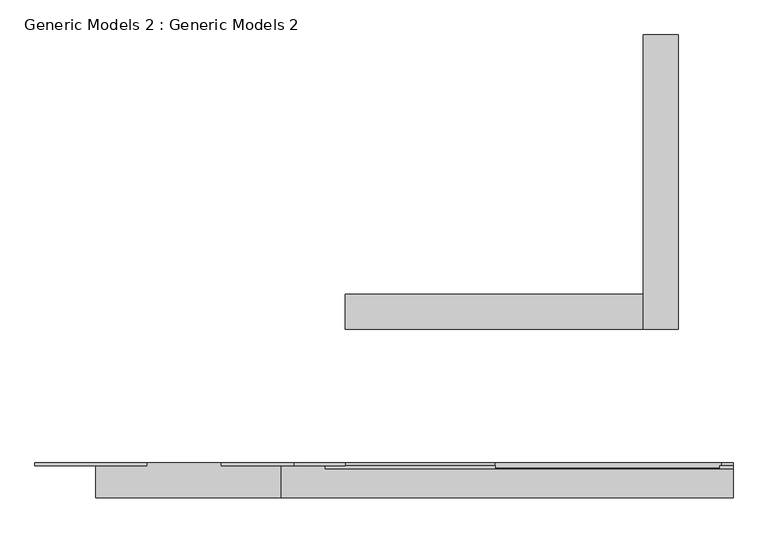
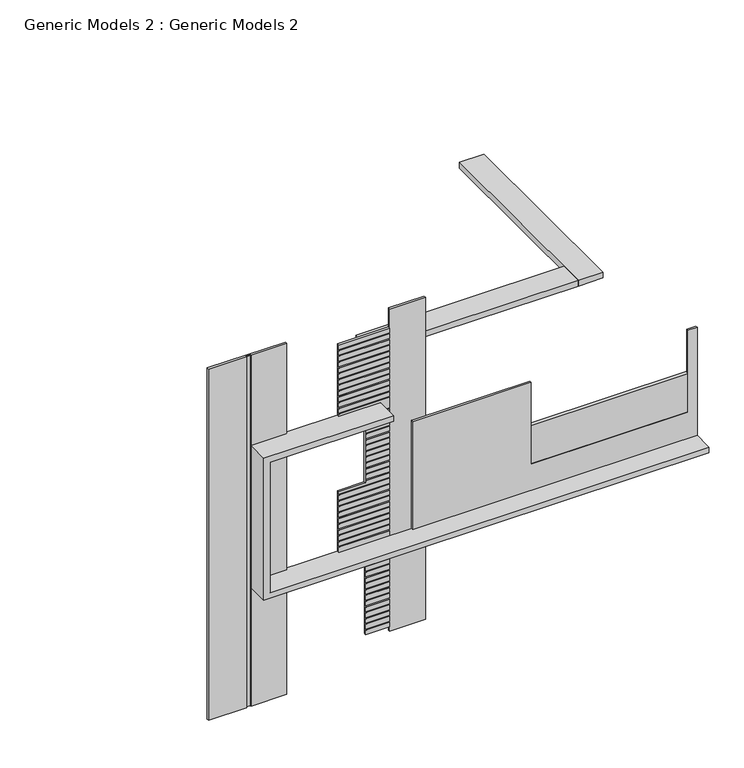
"""IFC4 building model written with IfcOpenShell, lengths in millimetres: proxy geometry, Generic Models 2 : Generic Models 2."""

from ifc_helpers import new_model, si_unit, frame, origin, place, context, project, spatial, polyline, outline, extrude, faceted_brep, source, transform, mapped, element, save


def generic_models_2_generic_models_2_2375a9c3(model_context):
    return source(origin(), model_context, "Body", "SolidModel", [
        faceted_brep([(-5276.7540309, 144.4033856, 8586.3008541), (-6547.458058, 144.4033856, 8586.3008541), (-6547.458058, 144.4033856, 8467.6502269), (-5276.7540309, 144.4033856, 8467.6502269), (-6547.458058, 144.4033856, 6705.6), (-5506.058058, 144.4033856, 6705.6), (-5506.058058, 144.4033856, 6553.2), (-5880.0040309, 144.4033856, 6553.2), (-5880.0040309, 144.4033856, 4724.4), (-6547.458058, 144.4033856, 4724.4), (-6547.458058, 144.4033856, 4660.9), (-5276.7540309, 144.4033856, 4660.9), (-5276.7540309, 144.4033856, 4724.4), (-5276.7540309, 144.4033856, 4783.2732683), (-5874.451629, 144.4033856, 4783.2732683), (-5874.451629, 144.4033856, 4813.3), (-5276.7540309, 144.4033856, 4813.3), (-5276.7540309, 144.4033856, 4935.6732683), (-5874.451629, 144.4033856, 4935.6732683), (-5874.451629, 144.4033856, 4965.7), (-5276.7540309, 144.4033856, 4965.7), (-5276.7540309, 144.4033856, 5088.0732683), (-5874.451629, 144.4033856, 5088.0732683), (-5874.451629, 144.4033856, 5118.1), (-5276.7540309, 144.4033856, 5118.1), (-5276.7540309, 144.4033856, 5240.4732683), (-5874.451629, 144.4033856, 5240.4732683), (-5874.451629, 144.4033856, 5270.5), (-5276.7540309, 144.4033856, 5270.5), (-5276.7540309, 144.4033856, 5392.8732683), (-5874.451629, 144.4033856, 5392.8732683), (-5874.451629, 144.4033856, 5422.9), (-5276.7540309, 144.4033856, 5422.9), (-5276.7540309, 144.4033856, 5545.2732683), (-5874.451629, 144.4033856, 5545.2732683), (-5874.451629, 144.4033856, 5575.3), (-5276.7540309, 144.4033856, 5575.3), (-5276.7540309, 144.4033856, 5697.6732683), (-5874.451629, 144.4033856, 5697.6732683), (-5874.451629, 144.4033856, 5727.7), (-5276.7540309, 144.4033856, 5727.7), (-5276.7540309, 144.4033856, 5850.0732683), (-5874.451629, 144.4033856, 5850.0732683), (-5874.451629, 144.4033856, 5880.1), (-5276.7540309, 144.4033856, 5880.1), (-5276.7540309, 144.4033856, 6002.4732683), (-5874.451629, 144.4033856, 6002.4732683), (-5874.451629, 144.4033856, 6032.5), (-5276.7540309, 144.4033856, 6032.5), (-5276.7540309, 144.4033856, 6154.8732683), (-5874.451629, 144.4033856, 6154.8732683), (-5874.451629, 144.4033856, 6184.9), (-5276.7540309, 144.4033856, 6184.9), (-5276.7540309, 144.4033856, 6307.2732683), (-5874.451629, 144.4033856, 6307.2732683), (-5874.451629, 144.4033856, 6337.3), (-5276.7540309, 144.4033856, 6337.3), (-5276.7540309, 144.4033856, 6459.6732683), (-5874.451629, 144.4033856, 6459.6732683), (-5874.451629, 144.4033856, 6489.7), (-5276.7540309, 144.4033856, 6489.7), (-5276.7540309, 144.4033856, 6761.2234952), (-6547.458058, 144.4033856, 6761.2234952), (-6547.458058, 144.4033856, 3124.2), (-5276.7540309, 144.4033856, 3124.2), (-5276.7540309, 144.4033856, 3259.2732683), (-6547.458058, 144.4033856, 3259.2732683), (-5276.7540309, 144.4033856, 8315.2502269), (-5276.7540309, 144.4033856, 8437.6234952), (-6547.458058, 144.4033856, 8437.6234952), (-6547.458058, 144.4033856, 8315.2502269), (-5276.7540309, 144.4033856, 8162.8502269), (-5276.7540309, 144.4033856, 8285.2234952), (-6547.458058, 144.4033856, 8285.2234952), (-6547.458058, 144.4033856, 8162.8502269), (-5276.7540309, 144.4033856, 8010.4502269), (-5276.7540309, 144.4033856, 8132.8234952), (-6547.458058, 144.4033856, 8132.8234952), (-6547.458058, 144.4033856, 8010.4502269), (-5276.7540309, 144.4033856, 7858.0502269), (-5276.7540309, 144.4033856, 7980.4234952), (-6547.458058, 144.4033856, 7980.4234952), (-6547.458058, 144.4033856, 7858.0502269), (-5276.7540309, 144.4033856, 7705.6502269), (-5276.7540309, 144.4033856, 7828.0234952), (-6547.458058, 144.4033856, 7828.0234952), (-6547.458058, 144.4033856, 7705.6502269), (-5276.7540309, 144.4033856, 7553.2502269), (-5276.7540309, 144.4033856, 7675.6234952), (-6547.458058, 144.4033856, 7675.6234952), (-6547.458058, 144.4033856, 7553.2502269), (-5276.7540309, 144.4033856, 7400.8502269), (-5276.7540309, 144.4033856, 7523.2234952), (-6547.458058, 144.4033856, 7523.2234952), (-6547.458058, 144.4033856, 7400.8502269), (-5276.7540309, 144.4033856, 7248.4502269), (-5276.7540309, 144.4033856, 7370.8234952), (-6547.458058, 144.4033856, 7370.8234952), (-6547.458058, 144.4033856, 7248.4502269), (-5276.7540309, 144.4033856, 7096.0502269), (-5276.7540309, 144.4033856, 7218.4234952), (-6547.458058, 144.4033856, 7218.4234952), (-6547.458058, 144.4033856, 7096.0502269), (-5276.7540309, 144.4033856, 6943.6502269), (-5276.7540309, 144.4033856, 7066.0234952), (-6547.458058, 144.4033856, 7066.0234952), (-6547.458058, 144.4033856, 6943.6502269), (-5276.7540309, 144.4033856, 6791.2502269), (-5276.7540309, 144.4033856, 6913.6234952), (-6547.458058, 144.4033856, 6913.6234952), (-6547.458058, 144.4033856, 6791.2502269), (-6547.458058, 144.4033856, 4630.8732683), (-6547.458058, 144.4033856, 4508.5), (-5276.7540309, 144.4033856, 4508.5), (-5276.7540309, 144.4033856, 4630.8732683), (-6547.458058, 144.4033856, 4478.4732683), (-6547.458058, 144.4033856, 4356.1), (-5276.7540309, 144.4033856, 4356.1), (-5276.7540309, 144.4033856, 4478.4732683), (-6547.458058, 144.4033856, 4326.0732683), (-6547.458058, 144.4033856, 4203.7), (-5276.7540309, 144.4033856, 4203.7), (-5276.7540309, 144.4033856, 4326.0732683), (-6547.458058, 144.4033856, 4173.6732683), (-6547.458058, 144.4033856, 4051.3), (-5276.7540309, 144.4033856, 4051.3), (-5276.7540309, 144.4033856, 4173.6732683), (-6547.458058, 144.4033856, 4021.2732683), (-6547.458058, 144.4033856, 3898.9), (-5276.7540309, 144.4033856, 3898.9), (-5276.7540309, 144.4033856, 4021.2732683), (-6547.458058, 144.4033856, 3868.8732683), (-6547.458058, 144.4033856, 3746.5), (-5276.7540309, 144.4033856, 3746.5), (-5276.7540309, 144.4033856, 3868.8732683), (-6547.458058, 144.4033856, 3716.4732683), (-6547.458058, 144.4033856, 3594.1), (-5276.7540309, 144.4033856, 3594.1), (-5276.7540309, 144.4033856, 3716.4732683), (-6547.458058, 144.4033856, 3564.0732683), (-6547.458058, 144.4033856, 3441.7), (-5276.7540309, 144.4033856, 3441.7), (-5276.7540309, 144.4033856, 3564.0732683), (-6547.458058, 144.4033856, 3411.6732683), (-6547.458058, 144.4033856, 3289.3), (-5276.7540309, 144.4033856, 3289.3), (-5276.7540309, 144.4033856, 3411.6732683), (-5276.7540309, 195.2033856, 4724.4), (-5276.7540309, 195.2033856, 3124.2), (-6547.458058, 195.2033856, 3124.2), (-6547.458058, 195.2033856, 4724.4), (-5880.0040309, 195.2033856, 4724.4), (-5880.0040309, 195.2033856, 6553.2), (-5506.058058, 195.2033856, 6553.2), (-5506.058058, 195.2033856, 6705.6), (-6547.458058, 195.2033856, 6705.6), (-6547.458058, 195.2033856, 8586.3008541), (-5276.7540309, 195.2033856, 8586.3008541), (-5276.7540309, 145.6932294, 8467.6502269), (-5276.7540309, 145.6932294, 8437.6234952), (-5276.7540309, 145.6932294, 8315.2502269), (-5276.7540309, 145.6932294, 8285.2234952), (-5276.7540309, 145.6932294, 8162.8502269), (-5276.7540309, 145.6932294, 8132.8234952), (-5276.7540309, 145.6932294, 8010.4502269), (-5276.7540309, 145.6932294, 7980.4234952), (-5276.7540309, 145.6932294, 7858.0502269), (-5276.7540309, 145.6932294, 7828.0234952), (-5276.7540309, 145.6932294, 7705.6502269), (-5276.7540309, 145.6932294, 7675.6234952), (-5276.7540309, 145.6932294, 7553.2502269), (-5276.7540309, 145.6932294, 7523.2234952), (-5276.7540309, 145.6932294, 7400.8502269), (-5276.7540309, 145.6932294, 7370.8234952), (-5276.7540309, 145.6932294, 7248.4502269), (-5276.7540309, 145.6932294, 7218.4234952), (-5276.7540309, 145.6932294, 7096.0502269), (-5276.7540309, 145.6932294, 7066.0234952), (-5276.7540309, 145.6932294, 6943.6502269), (-5276.7540309, 145.6932294, 6913.6234952), (-5276.7540309, 145.6932294, 6791.2502269), (-5276.7540309, 145.6932294, 6761.2234952), (-5276.7540309, 145.6932294, 6489.7), (-5276.7540309, 145.6932294, 6459.6732683), (-5276.7540309, 145.6932294, 6337.3), (-5276.7540309, 145.6932294, 6307.2732683), (-5276.7540309, 145.6932294, 6184.9), (-5276.7540309, 145.6932294, 6154.8732683), (-5276.7540309, 145.6932294, 6032.5), (-5276.7540309, 145.6932294, 6002.4732683), (-5276.7540309, 145.6932294, 5880.1), (-5276.7540309, 145.6932294, 5850.0732683), (-5276.7540309, 145.6932294, 5727.7), (-5276.7540309, 145.6932294, 5697.6732683), (-5276.7540309, 145.6932294, 5575.3), (-5276.7540309, 145.6932294, 5545.2732683), (-5276.7540309, 145.6932294, 5422.9), (-5276.7540309, 145.6932294, 5392.8732683), (-5276.7540309, 145.6932294, 5270.5), (-5276.7540309, 145.6932294, 5240.4732683), (-5276.7540309, 145.6932294, 5118.1), (-5276.7540309, 145.6932294, 5088.0732683), (-5276.7540309, 145.6932294, 4965.7), (-5276.7540309, 145.6932294, 4935.6732683), (-5276.7540309, 145.6932294, 4813.3), (-5276.7540309, 145.6932294, 4783.2732683), (-6547.458058, 145.6932294, 6761.2234952), (-6547.458058, 145.6932294, 6791.2502269), (-6547.458058, 145.6932294, 6913.6234952), (-6547.458058, 145.6932294, 6943.6502269), (-6547.458058, 145.6932294, 7066.0234952), (-6547.458058, 145.6932294, 7096.0502269), (-6547.458058, 145.6932294, 7218.4234952), (-6547.458058, 145.6932294, 7248.4502269), (-6547.458058, 145.6932294, 7370.8234952), (-6547.458058, 145.6932294, 7400.8502269), (-6547.458058, 145.6932294, 7523.2234952), (-6547.458058, 145.6932294, 7553.2502269), (-6547.458058, 145.6932294, 7675.6234952), (-6547.458058, 145.6932294, 7705.6502269), (-6547.458058, 145.6932294, 7828.0234952), (-6547.458058, 145.6932294, 7858.0502269), (-6547.458058, 145.6932294, 7980.4234952), (-6547.458058, 145.6932294, 8010.4502269), (-6547.458058, 145.6932294, 8132.8234952), (-6547.458058, 145.6932294, 8162.8502269), (-6547.458058, 145.6932294, 8285.2234952), (-6547.458058, 145.6932294, 8315.2502269), (-6547.458058, 145.6932294, 8437.6234952), (-6547.458058, 145.6932294, 8467.6502269), (-6547.458058, 145.6932294, 3259.2732683), (-6547.458058, 145.6932294, 3289.3), (-6547.458058, 145.6932294, 3411.6732683), (-6547.458058, 145.6932294, 3441.7), (-6547.458058, 145.6932294, 3564.0732683), (-6547.458058, 145.6932294, 3594.1), (-6547.458058, 145.6932294, 3716.4732683), (-6547.458058, 145.6932294, 3746.5), (-6547.458058, 145.6932294, 3868.8732683), (-6547.458058, 145.6932294, 3898.9), (-6547.458058, 145.6932294, 4021.2732683), (-6547.458058, 145.6932294, 4051.3), (-6547.458058, 145.6932294, 4173.6732683), (-6547.458058, 145.6932294, 4203.7), (-6547.458058, 145.6932294, 4326.0732683), (-6547.458058, 145.6932294, 4356.1), (-6547.458058, 145.6932294, 4478.4732683), (-6547.458058, 145.6932294, 4508.5), (-6547.458058, 145.6932294, 4630.8732683), (-6547.458058, 145.6932294, 4660.9), (-5276.7540309, 145.6932294, 4660.9), (-5276.7540309, 145.6932294, 4630.8732683), (-5276.7540309, 145.6932294, 4508.5), (-5276.7540309, 145.6932294, 4478.4732683), (-5276.7540309, 145.6932294, 4356.1), (-5276.7540309, 145.6932294, 4326.0732683), (-5276.7540309, 145.6932294, 4203.7), (-5276.7540309, 145.6932294, 4173.6732683), (-5276.7540309, 145.6932294, 4051.3), (-5276.7540309, 145.6932294, 4021.2732683), (-5276.7540309, 145.6932294, 3898.9), (-5276.7540309, 145.6932294, 3868.8732683), (-5276.7540309, 145.6932294, 3746.5), (-5276.7540309, 145.6932294, 3716.4732683), (-5276.7540309, 145.6932294, 3594.1), (-5276.7540309, 145.6932294, 3564.0732683), (-5276.7540309, 145.6932294, 3441.7), (-5276.7540309, 145.6932294, 3411.6732683), (-5276.7540309, 145.6932294, 3289.3), (-5276.7540309, 145.6932294, 3259.2732683), (-5874.451629, 145.6932294, 6459.6732683), (-5874.451629, 145.6932294, 6489.7), (-5874.451629, 145.6932294, 6307.2732683), (-5874.451629, 145.6932294, 6337.3), (-5874.451629, 145.6932294, 6154.8732683), (-5874.451629, 145.6932294, 6184.9), (-5874.451629, 145.6932294, 6002.4732683), (-5874.451629, 145.6932294, 6032.5), (-5874.451629, 145.6932294, 5850.0732683), (-5874.451629, 145.6932294, 5880.1), (-5874.451629, 145.6932294, 5697.6732683), (-5874.451629, 145.6932294, 5727.7), (-5874.451629, 145.6932294, 5545.2732683), (-5874.451629, 145.6932294, 5575.3), (-5874.451629, 145.6932294, 5392.8732683), (-5874.451629, 145.6932294, 5422.9), (-5874.451629, 145.6932294, 5240.4732683), (-5874.451629, 145.6932294, 5270.5), (-5874.451629, 145.6932294, 5088.0732683), (-5874.451629, 145.6932294, 5118.1), (-5874.451629, 145.6932294, 4935.6732683), (-5874.451629, 145.6932294, 4965.7), (-5874.451629, 145.6932294, 4783.2732683), (-5874.451629, 145.6932294, 4813.3)], [[[0, 1, 2, 3]], [[4, 5, 6, 7, 8, 9, 10, 11, 12, 13, 14, 15, 16, 17, 18, 19, 20, 21, 22, 23, 24, 25, 26, 27, 28, 29, 30, 31, 32, 33, 34, 35, 36, 37, 38, 39, 40, 41, 42, 43, 44, 45, 46, 47, 48, 49, 50, 51, 52, 53, 54, 55, 56, 57, 58, 59, 60, 61, 62]], [[63, 64, 65, 66]], [[67, 68, 69, 70]], [[71, 72, 73, 74]], [[75, 76, 77, 78]], [[79, 80, 81, 82]], [[83, 84, 85, 86]], [[87, 88, 89, 90]], [[91, 92, 93, 94]], [[95, 96, 97, 98]], [[99, 100, 101, 102]], [[103, 104, 105, 106]], [[107, 108, 109, 110]], [[111, 112, 113, 114]], [[115, 116, 117, 118]], [[119, 120, 121, 122]], [[123, 124, 125, 126]], [[127, 128, 129, 130]], [[131, 132, 133, 134]], [[135, 136, 137, 138]], [[139, 140, 141, 142]], [[143, 144, 145, 146]], [[147, 148, 149, 150, 151, 152, 153, 154, 155, 156, 157]], [[147, 157, 0, 3, 158, 159, 68, 67, 160, 161, 72, 71, 162, 163, 76, 75, 164, 165, 80, 79, 166, 167, 84, 83, 168, 169, 88, 87, 170, 171, 92, 91, 172, 173, 96, 95, 174, 175, 100, 99, 176, 177, 104, 103, 178, 179, 108, 107, 180, 181, 61, 60, 182, 183, 57, 56, 184, 185, 53, 52, 186, 187, 49, 48, 188, 189, 45, 44, 190, 191, 41, 40, 192, 193, 37, 36, 194, 195, 33, 32, 196, 197, 29, 28, 198, 199, 25, 24, 200, 201, 21, 20, 202, 203, 17, 16, 204, 205, 13, 12]], [[1, 0, 157, 156]], [[156, 155, 4, 62, 206, 207, 110, 109, 208, 209, 106, 105, 210, 211, 102, 101, 212, 213, 98, 97, 214, 215, 94, 93, 216, 217, 90, 89, 218, 219, 86, 85, 220, 221, 82, 81, 222, 223, 78, 77, 224, 225, 74, 73, 226, 227, 70, 69, 228, 229, 2, 1]], [[5, 4, 155, 154]], [[6, 5, 154, 153]], [[7, 6, 153, 152]], [[8, 7, 152, 151]], [[9, 8, 151, 150]], [[150, 149, 63, 66, 230, 231, 144, 143, 232, 233, 140, 139, 234, 235, 136, 135, 236, 237, 132, 131, 238, 239, 128, 127, 240, 241, 124, 123, 242, 243, 120, 119, 244, 245, 116, 115, 246, 247, 112, 111, 248, 249, 10, 9]], [[64, 63, 149, 148]], [[148, 147, 12, 11, 250, 251, 114, 113, 252, 253, 118, 117, 254, 255, 122, 121, 256, 257, 126, 125, 258, 259, 130, 129, 260, 261, 134, 133, 262, 263, 138, 137, 264, 265, 142, 141, 266, 267, 146, 145, 268, 269, 65, 64]], [[228, 159, 158, 229]], [[226, 161, 160, 227]], [[224, 163, 162, 225]], [[222, 165, 164, 223]], [[220, 167, 166, 221]], [[218, 169, 168, 219]], [[216, 171, 170, 217]], [[214, 173, 172, 215]], [[212, 175, 174, 213]], [[210, 177, 176, 211]], [[208, 179, 178, 209]], [[206, 181, 180, 207]], [[270, 183, 182, 271]], [[272, 185, 184, 273]], [[274, 187, 186, 275]], [[276, 189, 188, 277]], [[278, 191, 190, 279]], [[280, 193, 192, 281]], [[282, 195, 194, 283]], [[284, 197, 196, 285]], [[286, 199, 198, 287]], [[288, 201, 200, 289]], [[290, 203, 202, 291]], [[292, 205, 204, 293]], [[248, 251, 250, 249]], [[246, 253, 252, 247]], [[244, 255, 254, 245]], [[242, 257, 256, 243]], [[240, 259, 258, 241]], [[238, 261, 260, 239]], [[236, 263, 262, 237]], [[234, 265, 264, 235]], [[232, 267, 266, 233]], [[230, 269, 268, 231]], [[229, 158, 3, 2]], [[159, 228, 69, 68]], [[227, 160, 67, 70]], [[161, 226, 73, 72]], [[225, 162, 71, 74]], [[163, 224, 77, 76]], [[223, 164, 75, 78]], [[165, 222, 81, 80]], [[221, 166, 79, 82]], [[167, 220, 85, 84]], [[219, 168, 83, 86]], [[169, 218, 89, 88]], [[217, 170, 87, 90]], [[171, 216, 93, 92]], [[215, 172, 91, 94]], [[173, 214, 97, 96]], [[213, 174, 95, 98]], [[175, 212, 101, 100]], [[211, 176, 99, 102]], [[177, 210, 105, 104]], [[209, 178, 103, 106]], [[179, 208, 109, 108]], [[207, 180, 107, 110]], [[181, 206, 62, 61]], [[270, 271, 59, 58]], [[271, 182, 60, 59]], [[183, 270, 58, 57]], [[272, 273, 55, 54]], [[273, 184, 56, 55]], [[185, 272, 54, 53]], [[274, 275, 51, 50]], [[275, 186, 52, 51]], [[187, 274, 50, 49]], [[276, 277, 47, 46]], [[277, 188, 48, 47]], [[189, 276, 46, 45]], [[278, 279, 43, 42]], [[279, 190, 44, 43]], [[191, 278, 42, 41]], [[280, 281, 39, 38]], [[281, 192, 40, 39]], [[193, 280, 38, 37]], [[282, 283, 35, 34]], [[283, 194, 36, 35]], [[195, 282, 34, 33]], [[284, 285, 31, 30]], [[285, 196, 32, 31]], [[197, 284, 30, 29]], [[286, 287, 27, 26]], [[287, 198, 28, 27]], [[199, 286, 26, 25]], [[288, 289, 23, 22]], [[289, 200, 24, 23]], [[201, 288, 22, 21]], [[290, 291, 19, 18]], [[291, 202, 20, 19]], [[203, 290, 18, 17]], [[292, 293, 15, 14]], [[293, 204, 16, 15]], [[205, 292, 14, 13]], [[249, 250, 11, 10]], [[251, 248, 111, 114]], [[247, 252, 113, 112]], [[253, 246, 115, 118]], [[245, 254, 117, 116]], [[255, 244, 119, 122]], [[243, 256, 121, 120]], [[257, 242, 123, 126]], [[241, 258, 125, 124]], [[259, 240, 127, 130]], [[239, 260, 129, 128]], [[261, 238, 131, 134]], [[237, 262, 133, 132]], [[263, 236, 135, 138]], [[235, 264, 137, 136]], [[265, 234, 139, 142]], [[233, 266, 141, 140]], [[267, 232, 143, 146]], [[231, 268, 145, 144]], [[269, 230, 66, 65]]]),
        extrude(outline(polyline([(195.2033856, 2971.8), (195.2033856, 733.1770356), (144.4033856, 733.1770356), (144.4033856, 846.2732683), (145.6932294, 846.2732683), (145.6932294, 876.3), (144.4033856, 876.3), (144.4033856, 998.6732683), (145.6932294, 998.6732683), (145.6932294, 1028.7), (144.4033856, 1028.7), (144.4033856, 1151.0732683), (145.6932294, 1151.0732683), (145.6932294, 1181.1), (144.4033856, 1181.1), (144.4033856, 1303.4732683), (145.6932294, 1303.4732683), (145.6932294, 1333.5), (144.4033856, 1333.5), (144.4033856, 1455.8732683), (145.6932294, 1455.8732683), (145.6932294, 1485.9), (144.4033856, 1485.9), (144.4033856, 1608.2732683), (145.6932294, 1608.2732683), (145.6932294, 1638.3), (144.4033856, 1638.3), (144.4033856, 1760.6732683), (145.6932294, 1760.6732683), (145.6932294, 1790.7), (144.4033856, 1790.7), (144.4033856, 1913.0732683), (145.6932294, 1913.0732683), (145.6932294, 1943.1), (144.4033856, 1943.1), (144.4033856, 2065.4732683), (145.6932294, 2065.4732683), (145.6932294, 2095.5), (144.4033856, 2095.5), (144.4033856, 2217.8732683), (145.6932294, 2217.8732683), (145.6932294, 2247.9), (144.4033856, 2247.9), (144.4033856, 2370.2732683), (145.6932294, 2370.2732683), (145.6932294, 2400.3), (144.4033856, 2400.3), (144.4033856, 2522.6732683), (145.6932294, 2522.6732683), (145.6932294, 2552.7), (144.4033856, 2552.7), (144.4033856, 2675.0732683), (145.6932294, 2675.0732683), (145.6932294, 2705.1), (144.4033856, 2705.1), (144.4033856, 2827.4732683), (145.6932294, 2827.4732683), (145.6932294, 2857.5), (144.4033856, 2857.5), (144.4033856, 2971.8), (195.2033856, 2971.8)])), frame((-5874.451629, 0.0, 0.0), z_axis=(1.0, 0.0, 0.0), x_axis=(0.0, 1.0, 0.0)), (0.0, 0.0, 1.0), 597.6975981),
        extrude(outline(polyline([(-4387.7540309, 144.4033856), (-5276.7540309, 144.4033856), (-5276.7540309, 195.2033856), (-4387.7540309, 195.2033856), (-4387.7540309, 144.4033856)])), frame((0.0, 0.0, 609.6), z_axis=(0.0, 0.0, 1.0), x_axis=(1.0, 0.0, 0.0)), (0.0, 0.0, 1.0), 8478.1987802),
        faceted_brep([(-7840.4748309, 144.4033856, -152.4), (-7840.4748309, 144.4033856, 9087.7987802), (-9785.2540309, 144.4033856, 9087.7987802), (-9785.2540309, 144.4033856, -152.4), (-8832.7540309, 144.4033856, -152.4), (-8832.7540309, 144.4033856, 9086.85), (-8731.1540309, 144.4033856, 9086.85), (-8731.1540309, 144.4033856, -152.4), (-9785.2540309, 195.2033856, -152.4), (-9785.2540309, 195.2033856, 9087.7987802), (-7840.4748309, 195.2033856, 9087.7987802), (-7840.4748309, 195.2033856, -152.4), (-8731.1540309, 169.8033856, -152.4), (-8832.7540309, 169.8033856, -152.4), (-8832.7540309, 169.8033856, 9086.85), (-8731.1540309, 169.8033856, 9086.85)], [[[0, 1, 2, 3, 4, 5, 6, 7]], [[8, 9, 10, 11]], [[8, 11, 0, 7, 12, 13, 4, 3]], [[1, 0, 11, 10]], [[2, 1, 10, 9]], [[3, 2, 9, 8]], [[14, 13, 12, 15]], [[14, 15, 6, 5]], [[15, 12, 7, 6]], [[13, 14, 5, 4]]]),
        extrude(outline(polyline([(2971.8, 2355.9459691), (3124.2, 2355.9459691), (3124.2, -8578.7540309), (6553.2, -8578.7540309), (6553.2, -5506.058058), (6705.6, -5506.058058), (6705.6, -8731.1540309), (2971.8, -8731.1540309), (2971.8, 2355.9459691)])), frame((0.0, -414.3966144, 0.0), z_axis=(0.0, 1.0, 0.0), x_axis=(0.0, 0.0, 1.0)), (0.0, 0.0, 1.0), 609.6),
        extrude(outline(polyline([(2152.7459691, 195.2033856), (2152.7459691, 112.6533856), (-1784.2540309, 112.6533856), (-1784.2540309, 195.2033856), (2152.7459691, 195.2033856)])), frame((0.0, 0.0, 3809.8487325), z_axis=(0.0, 0.0, 1.0), x_axis=(1.0, 0.0, 0.0)), (0.0, 0.0, 1.0), 1009.8012675),
        extrude(outline(polyline([(3124.2, -4735.2247224), (3124.2, 2355.9459691), (5969.0, 2355.9459691), (5969.0, 2127.3459691), (3810.0, 2127.3459691), (3810.0, -1784.2540309), (5969.0, -1784.2540309), (5969.0, -4735.2247224), (3124.2, -4735.2247224)])), frame((0.0, 93.6033856, 0.0), z_axis=(0.0, 1.0, 0.0), x_axis=(0.0, 0.0, 1.0)), (0.0, 0.0, 1.0), 50.8),
        extrude(outline(polyline([(1403.4459691, 7634.9360044), (1403.4459691, 2519.3033856), (793.8459691, 2519.3033856), (793.8459691, 7634.9360044), (1403.4459691, 7634.9360044)])), frame((0.0, 0.0, 6129.0490524), z_axis=(0.0, 0.0, 1.0), x_axis=(1.0, 0.0, 0.0)), (0.0, 0.0, 1.0), 152.4),
        extrude(outline(polyline([(793.8459691, 2519.3033856), (-4387.7540309, 2519.3033856), (-4387.7540309, 3128.9033856), (793.8459691, 3128.9033856), (793.8459691, 2519.3033856)])), frame((0.0, 0.0, 6129.0490524), z_axis=(0.0, 0.0, 1.0), x_axis=(1.0, 0.0, 0.0)), (0.0, 0.0, 1.0), 152.4),
    ])


if __name__ == "__main__":
    model = new_model("IFC4")
    model_context = context("Model", 3, world=origin())
    ifc_project = project(units=[si_unit("LENGTHUNIT", "METRE", prefix="MILLI")], contexts=[model_context])
    site = spatial("IfcSite", under=ifc_project)
    building = spatial("IfcBuilding", under=site)
    placement = place(None, origin())
    generic_models_2_generic_models_2_shape = generic_models_2_generic_models_2_2375a9c3(model_context)
    element("IfcBuildingElementProxy", 1, Name="Generic Models 2 : Generic Models 2", ObjectType="Generic Models 2 : Generic Models 2", at=placement, inside=building, context=model_context, shape_type="MappedRepresentation", body=[
        mapped(generic_models_2_generic_models_2_shape, transform((0.0, 0.0, 0.0), x_axis=(1.0, 0.0, 0.0), y_axis=(0.0, 1.0, 0.0), z_axis=(0.0, 0.0, 1.0))),
    ])
    save(model, "model.ifc")

# Revit data of these elements
# Element 1 (IfcBuildingElementProxy, "Generic Models 2 : Generic Models 2")
#   Materials on its faces: "Gypsum Wall Board", "Laminate, Ivory, Matte"
# Materials
#   "Gypsum Wall Board": class "Generic", colour RGB 127 127 127, transparency 0, Description = "Gypsum Wall Board", Cost = 0
#   "Laminate, Ivory, Matte": class "Plastic", colour RGB 247 247 239, transparency 0, Description = "Plastic Laminate - Ivory, Matte", Cost = 0
